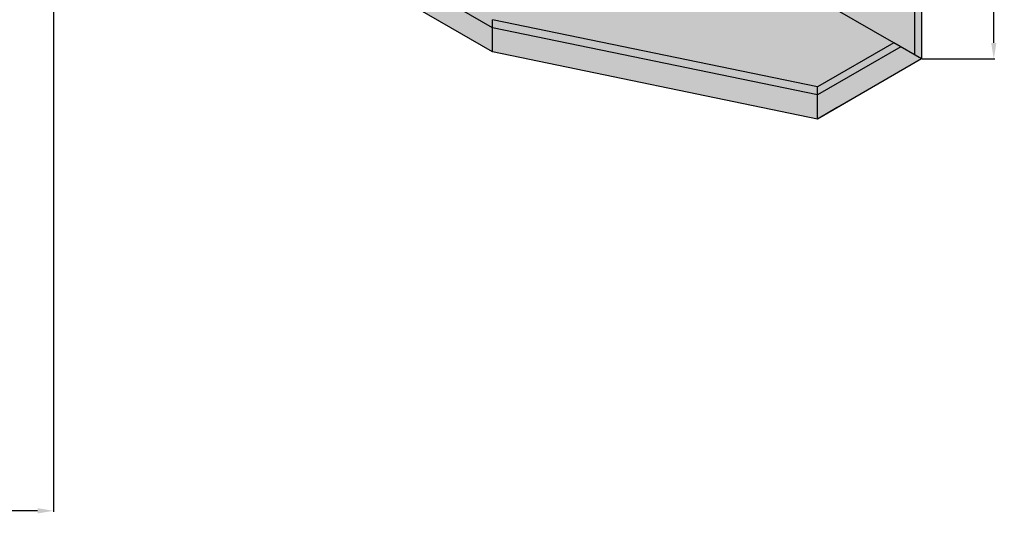
# Model space of a CAD drawing. Units: millimetres. Extents: x 78378 to 86415, y 148682 to 152721.
# Tile 9 of 18: x 80650 to 81878, y 148682 to 149308. Entities that reach past the tile are written whole.
import ezdxf

# ---------------------------------------------------------------- set-up
doc = ezdxf.new("R2010")
doc.units = ezdxf.units.MM
for name, color, linetype, lineweight in [('A-ANNO-DIMS', 2, 'Continuous', 18), ('A-FURN', 4, 'Continuous', 25), ('A-FURN-PATT', 32, 'Continuous', 13)]:
    doc.layers.add(name, color=color, linetype=linetype, lineweight=lineweight)
doc.styles.get("Standard").update_dxf_attribs({"font": 'arial.ttf'})
doc.dimstyles.new('ISO-25', dxfattribs={"dimtxt": 20, "dimasz": 20, "dimexe": 1.25, "dimexo": 0.625, "dimtad": 0, "dimdec": 1, "dimtxsty": 'Standard', "dimcen": 2.5, "dimadec": 0, "dimazin": 0, "dimtfac": 1, "dimtdec": 1, "dimtmove": 0, "dimatfit": 3, "dimfxl": 1, "dimarcsym": 0})

# ---------------------------------------------------------------- blocks, each defined once
blk = doc.blocks.new('*D1')
at = {"layer": 'A-ANNO-DIMS', "color": 0, "lineweight": -2, "transparency": 16777216}
for p, q in [((81775.8, 151435), (81866.6, 151435)), ((81865.3, 151415), (81865.3, 150363.7)), ((81865.3, 149279), (81865.3, 150302.4)), ((81775.8, 149259), (81866.6, 149259))]:
    blk.add_line(p, q, dxfattribs=at)
at = {"layer": 'A-ANNO-DIMS', "color": 0, "transparency": 16777216}
for points in [[(81862, 151415), (81868.6, 151415), (81865.3, 151435)], [(81862, 149279), (81868.6, 149279), (81865.3, 149259)]]:
    blk.add_solid(points, dxfattribs=at)
at = {"layer": 'Defpoints', "color": 0, "transparency": 16777216}
for p in [(81775.2, 151435), (81775.2, 149259), (81865.3, 149259)]:
    blk.add_point(p, dxfattribs=at)
at = {"layer": 'A-ANNO-DIMS', "color": 0, "transparency": 16777216, "insert": (81865.3, 150333), "char_height": 20, "attachment_point": 5, "rotation": 90}
blk.add_mtext('2176', dxfattribs=at)
blk = doc.blocks.new('*D32')
at = {"layer": 'A-ANNO-DIMS', "color": 0, "lineweight": -2, "transparency": 16777216}
for p, q in [((80086.4, 150459.4), (80086.4, 148693.8)), ((80692.6, 150459.4), (80692.6, 148693.8)), ((80106.4, 148695), (80355.2, 148695)), ((80672.6, 148695), (80423.8, 148695))]:
    blk.add_line(p, q, dxfattribs=at)
at = {"layer": 'A-ANNO-DIMS', "color": 0, "transparency": 16777216}
for points in [[(80106.4, 148698.3), (80106.4, 148691.7), (80086.4, 148695)], [(80672.6, 148698.3), (80672.6, 148691.7), (80692.6, 148695)]]:
    blk.add_solid(points, dxfattribs=at)
at = {"layer": 'Defpoints', "color": 0, "transparency": 16777216}
for p in [(80086.4, 150460), (80692.6, 150460), (80692.6, 148695)]:
    blk.add_point(p, dxfattribs=at)
at = {"layer": 'A-ANNO-DIMS', "color": 0, "transparency": 16777216, "insert": (80389.5, 148695), "char_height": 20, "attachment_point": 5}
blk.add_mtext('606.2', dxfattribs=at)

msp = doc.modelspace()

# ---------------------------------------------------------------- hatches: boundary and pattern name
at = {"layer": 'A-FURN-PATT'}
h = msp.add_hatch(color=256, dxfattribs=at)
h.dxf.hatch_style = 1
h.paths.add_polyline_path([(81239.9694, 149691.4023), (81125.6347, 149757.4135), (81125.6347, 149727.4135), (81239.9694, 149661.4023), (81645.2499, 149577.4135), (81670.0493, 149591.7314), (81766.4935, 149647.4135), (81766.4935, 149657.4135), (81749.173, 149667.4135), (81645.2499, 149607.4135)])
h.paths.add_polyline_path([(81239.9694, 149701.4023), (81125.6347, 149767.4135), (81125.6347, 149757.4135), (81239.9694, 149691.4023), (81645.2499, 149607.4135), (81749.173, 149667.4135), (81740.5127, 149672.4135), (81645.2499, 149617.4135)])
h.paths.add_polyline_path([(81116.9744, 150195.0076), (80692.622, 150440.0076), (80692.622, 149614.0076), (81116.9744, 149369.0076)])
h.paths.add_polyline_path([(81073.6732, 149444.0076), (80735.9233, 149639.0076), (80735.9233, 150365.0076), (81073.6732, 150170.0076)], flags=16)
h.paths.add_polyline_path([(81125.6347, 149727.4135), (81116.9744, 149732.4135), (81116.9744, 149369.0076), (81239.9694, 149297.9965), (81239.9694, 149307.9965), (81125.6347, 149374.0076)])
h.paths.add_polyline_path([(81445.5517, 150047.7769), (81361.2342, 150053.9842), (81125.6347, 150190.0076), (81125.6347, 149767.4135), (81445.5517, 149842.7093)])
h.paths.add_polyline_path([(81239.9694, 149307.9965), (81239.9694, 149297.9965), (81645.2499, 149214.0076), (81645.2499, 149224.0076)])
h.paths.add_polyline_path([(81749.173, 149274.0076), (81740.5127, 149279.0076), (81645.2499, 149224.0076), (81645.2499, 149214.0076)])
h = msp.add_hatch(color=256, dxfattribs=at)
h.dxf.hatch_style = 1
h.paths.add_polyline_path([(81775.1537, 150105.0076), (81766.4935, 150100.0076), (81766.4935, 149657.4135), (81775.1537, 149652.4135)])
h.paths.add_polyline_path([(81775.1537, 149652.4135), (81766.4935, 149647.4135), (81766.4935, 149264.0076), (81775.1537, 149259.0076)])
h.paths.add_polyline_path([(81766.4935, 149657.4135), (81766.4935, 149647.4135), (81775.1537, 149652.4135)])
h = msp.add_hatch(color=256, dxfattribs=at)
h.dxf.hatch_style = 1
h.paths.add_polyline_path([(81445.5517, 149618.7982), (81239.9694, 149661.4023), (81125.6347, 149727.4135), (81125.6347, 149374.0076), (81445.5517, 149449.3035)])
h.paths.add_polyline_path([(81766.4935, 149647.4135), (81670.0493, 149591.7314), (81645.2499, 149577.4135), (81445.5517, 149618.7982), (81445.5517, 149449.3035), (81740.5127, 149279.0076), (81766.4935, 149264.0076)])
h.paths.add_polyline_path([(81445.5517, 149449.3035), (81125.6347, 149374.0076), (81239.9694, 149307.9965), (81645.2499, 149224.0076), (81740.5127, 149279.0076)])
h.paths.add_polyline_path([(81239.9694, 149297.9965), (81239.9694, 149267.9965), (81645.2499, 149184.0076), (81645.2499, 149214.0076)])
h = msp.add_hatch(color=256, dxfattribs=at)
h.dxf.hatch_style = 1
h.paths.add_polyline_path([(80086.4042, 149600.0076), (80692.622, 149584.0076), (81239.9694, 149267.9965), (81239.9694, 149297.9965), (81116.9744, 149369.0076), (80692.622, 149614.0076), (80086.4042, 149630.0076), (78830.6674, 148905.0076), (78830.6674, 148875.0076)])
h = msp.add_hatch(color=256, dxfattribs=at)
h.dxf.hatch_style = 1
h.paths.add_polyline_path([(81775.1537, 149259.0076), (81749.173, 149274.0076), (81645.2499, 149214.0076), (81645.2499, 149184.0076)])

# ---------------------------------------------------------------- linework, layer by layer
at = {"layer": 'A-FURN'}
for p, q in [((81775.1537, 151455.0076), (81775.1537, 149259.0076)), ((81766.4935, 151440.0076), (81766.4935, 149264.0076)), ((81239.9694, 149297.9965), (80692.622, 149614.0076)), ((81239.9694, 149267.9965), (80692.622, 149584.0076)), ((81740.5127, 149279.0076), (81445.5517, 149449.3035)), ((81239.9694, 149297.9965), (81116.9744, 149369.0076)), ((81645.2499, 149224.0076), (81239.9694, 149307.9965)), ((81239.9694, 149267.9965), (81239.9694, 149307.9965)), ((81645.2499, 149214.0076), (81239.9694, 149297.9965)), ((81740.5127, 149279.0076), (81645.2499, 149224.0076)), ((81775.1537, 149259.0076), (81740.5127, 149279.0076)), ((81645.2499, 149184.0076), (81239.9694, 149267.9965)), ((81749.173, 149274.0076), (81645.2499, 149214.0076)), ((81749.173, 149274.0076), (81645.2499, 149214.0076)), ((81775.1537, 149259.0076), (81645.2499, 149184.0076)), ((81775.1537, 149259.0076), (81670.0493, 149198.3255)), ((81645.2499, 149184.0076), (81645.2499, 149224.0076)), ((81670.0493, 149198.3255), (81645.2499, 149184.0076))]:
    msp.add_line(p, q, dxfattribs=at)

# ---------------------------------------------------------------- dimensions: what is measured, and where the dimension line sits
at = {"layer": 'A-ANNO-DIMS'}
dim = msp.add_linear_dim(base=(81865.3079, 149259.0076), p1=(81775.1537, 151435.0076), p2=(81775.1537, 149259.0076), angle=270, dimstyle='ISO-25', override={"dimclrd": 0, "dimclre": 0, "dimclrt": 0}, dxfattribs=at)
dim.commit()
dim.dimension.update_dxf_attribs({"geometry": '*D1', "text_midpoint": (81865.3079, 150333.0085), "dimtype": 161})
dim = msp.add_linear_dim(base=(80692.622, 148695.0076), p1=(80086.4042, 150460.0076), p2=(80692.622, 150460.0076), dimstyle='ISO-25', override={"dimdec": 1, "dimlfac": 1, "dimrnd": 0, "dimzin": 0, "dimdsep": 46, "dimlunit": 2}, dxfattribs=at)
dim.commit()
dim.dimension.update_dxf_attribs({"geometry": '*D32', "text_midpoint": (80389.5131, 148695.0076)})

doc.saveas('drawing.dxf')
